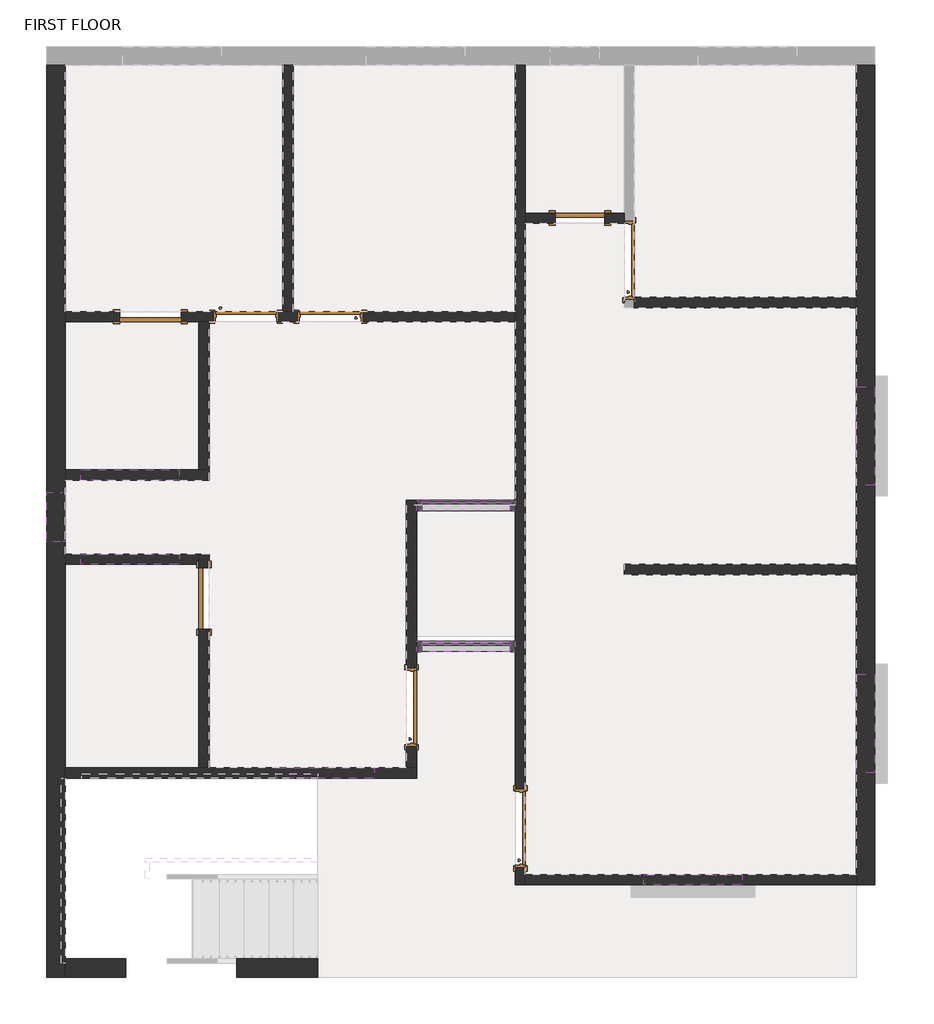
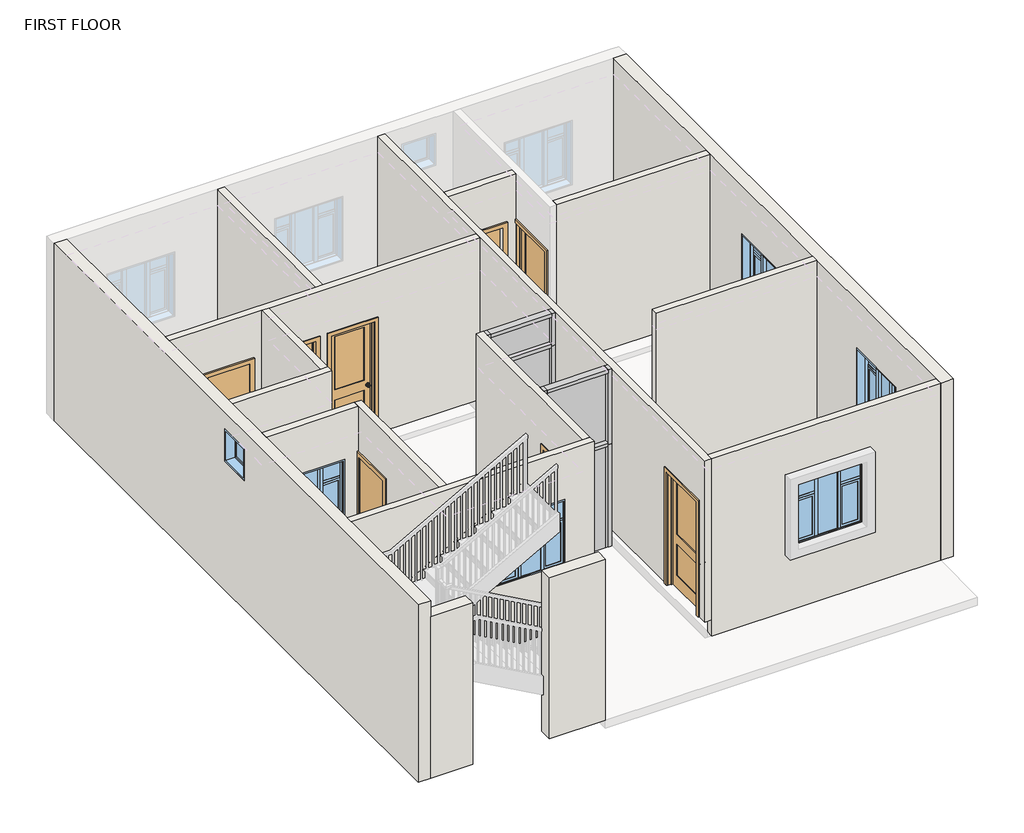
# One storey, part 1 of 3: 16 walls, 14 members, 8 doors, 7 windows, 4 plates.
"""IFC4 building model written with IfcOpenShell, lengths in millimetres."""

from ifc_helpers import new_model, si_unit, frame, origin, place, context, project, spatial, polyline, outline, extrude, faceted_brep, transform, mapped, element, save
from components import door_2e56f206, door_interior_single_2_panel_wood_main_doors_a5f98f63, door_interior_single_2_panel_wood_main_doors_4d656947, single_flush_bathroom_flush_door_4d6c7550, single_flush_bathroom_flush_door_2_931cabab, member_273a15f2, member_867fe1e1, member_ee409385, member_47bfaf8a, member_4b717c4e, system_panel_glazed_c5a9eb28, system_panel_glazed_3290db12, system_panel_glazed_e6353eef, fixed_opening_window_2_x_2_e119d648, window_casement_triple_side_transom_window_4_x_4_fd24aed3, window_casement_triple_side_transom_window_4_x_4_9406f89d

model = new_model("IFC4")

# Units and contexts
model_context = context("Model", 3, world=origin())
ifc_project = project(units=[si_unit("LENGTHUNIT", "METRE", prefix="MILLI")], contexts=[model_context])

# Site, building, storey
site = spatial("IfcSite", under=ifc_project)
building = spatial("IfcBuilding", under=site)
storey = spatial("IfcBuildingStorey", under=building, Name="FIRST FLOOR", Elevation=3352.8)

# Doors
placement = place(None, origin())
door_shape = door_2e56f206(model_context)
element("IfcDoor", 1, ObjectType="Door-Interior-Single-2_Panel-Wood : 36\" x 84\"", at=placement, inside=storey, context=model_context, shape_type="MappedRepresentation", body=[
    mapped(door_shape, transform((-9131.4273867, -1143.8499863, 3657.6), x_axis=(0.0, 1.0, 0.0), y_axis=(-1.0, 0.0, 0.0), z_axis=(0.0, 0.0, 1.0))),
])
element("IfcDoor", 2, ObjectType="Door-Interior-Single-2_Panel-Wood : 36\" x 84\"", at=placement, inside=storey, context=model_context, shape_type="MappedRepresentation", body=[
    mapped(door_shape, transform((-10477.6273867, 354.7500137, 3657.6), x_axis=(0.0, 1.0, 0.0), y_axis=(-1.0, 0.0, 0.0), z_axis=(0.0, 0.0, 1.0))),
])
element("IfcDoor", 3, ObjectType="Door-Interior-Single-2_Panel-Wood : 36\" x 84\"", at=placement, inside=storey, context=model_context, shape_type="MappedRepresentation", body=[
    mapped(door_shape, transform((-7785.2273867, 5879.2500137, 3657.6), x_axis=(0.0, 1.0, 0.0), y_axis=(-1.0, 0.0, 0.0), z_axis=(0.0, 0.0, 1.0))),
])
door_interior_single_2_panel_wood_main_doors_shape = door_interior_single_2_panel_wood_main_doors_a5f98f63(model_context)
element("IfcDoor", 4, ObjectType="Door-Interior-Single-2_Panel-Wood : MAIN DOORS", at=placement, inside=storey, context=model_context, shape_type="MappedRepresentation", body=[
    mapped(door_interior_single_2_panel_wood_main_doors_shape, transform((-12525.5023867, 5183.9250137, 3657.6), x_axis=(1.0, 0.0, 0.0), y_axis=(0.0, 1.0, 0.0), z_axis=(0.0, 0.0, 1.0))),
])
door_interior_single_2_panel_wood_main_doors_2_shape = door_interior_single_2_panel_wood_main_doors_4d656947(model_context)
element("IfcDoor", 5, ObjectType="Door-Interior-Single-2_Panel-Wood : MAIN DOORS", at=placement, inside=storey, context=model_context, shape_type="MappedRepresentation", body=[
    mapped(door_interior_single_2_panel_wood_main_doors_2_shape, transform((-11484.1023867, 5183.9250137, 3657.6), x_axis=(-1.0, 0.0, 0.0), y_axis=(0.0, -1.0, 0.0), z_axis=(0.0, 0.0, 1.0))),
])
single_flush_bathroom_flush_door_shape = single_flush_bathroom_flush_door_4d6c7550(model_context)
element("IfcDoor", 6, ObjectType="Single-Flush : BATHROOM FLUSH DOOR", at=placement, inside=storey, context=model_context, shape_type="MappedRepresentation", body=[
    mapped(single_flush_bathroom_flush_door_shape, transform((-13046.2023867, 1700.5265627, 3657.6), x_axis=(0.0, 1.0, 0.0), y_axis=(-1.0, 0.0, 0.0), z_axis=(0.0, 0.0, 1.0))),
])
element("IfcDoor", 7, ObjectType="Single-Flush : BATHROOM FLUSH DOOR", at=placement, inside=storey, context=model_context, shape_type="MappedRepresentation", body=[
    mapped(single_flush_bathroom_flush_door_shape, transform((-13706.6023867, 5180.7500137, 3657.6), x_axis=(-1.0, 0.0, 0.0), y_axis=(0.0, -1.0, 0.0), z_axis=(0.0, 0.0, 1.0))),
])
single_flush_bathroom_flush_door_2_shape = single_flush_bathroom_flush_door_2_931cabab(model_context)
element("IfcDoor", 8, ObjectType="Single-Flush : BATHROOM FLUSH DOOR 2", at=placement, inside=storey, context=model_context, shape_type="MappedRepresentation", body=[
    mapped(single_flush_bathroom_flush_door_2_shape, transform((-8398.0023867, 6399.9500137, 3657.6), x_axis=(-1.0, 0.0, 0.0), y_axis=(0.0, -1.0, 0.0), z_axis=(0.0, 0.0, 1.0))),
])

# Members
member_shape = member_273a15f2(model_context)
element("IfcMember", 9, ObjectType="Rectangular Mullion : 2.5\" x 5\" rectangular", at=placement, inside=storey, context=model_context, shape_type="MappedRepresentation", body=[
    mapped(member_shape, transform((-9261.6023867, 2848.1833471, 6705.6), x_axis=(0.0, 0.0, 1.0), y_axis=(0.0, -1.0, 0.0), z_axis=(1.0, 0.0, 0.0))),
])
element("IfcMember", 10, ObjectType="Rectangular Mullion : 2.5\" x 5\" rectangular", at=placement, inside=storey, context=model_context, shape_type="MappedRepresentation", body=[
    mapped(member_shape, transform((-9261.6023867, 1104.0500137, 6705.6), x_axis=(0.0, 0.0, 1.0), y_axis=(0.0, -1.0, 0.0), z_axis=(1.0, 0.0, 0.0))),
])
element("IfcMember", 11, ObjectType="Rectangular Mullion : 2.5\" x 5\" rectangular", at=placement, inside=storey, context=model_context, shape_type="MappedRepresentation", body=[
    mapped(member_shape, transform((-10353.8023867, 2848.1833471, 3657.6), x_axis=(0.0, 0.0, -1.0), y_axis=(0.0, -1.0, 0.0), z_axis=(-1.0, 0.0, 0.0))),
])
element("IfcMember", 12, ObjectType="Rectangular Mullion : 2.5\" x 5\" rectangular", at=placement, inside=storey, context=model_context, shape_type="MappedRepresentation", body=[
    mapped(member_shape, transform((-10353.8023867, 1104.0500137, 2851.15), x_axis=(0.0, 0.0, -1.0), y_axis=(0.0, -1.0, 0.0), z_axis=(-1.0, 0.0, 0.0))),
])
member_2_shape = member_867fe1e1(model_context)
element("IfcMember", 13, ObjectType="Rectangular Mullion : 2.5\" x 5\" rectangular", at=placement, inside=storey, context=model_context, shape_type="MappedRepresentation", body=[
    mapped(member_2_shape, transform((-9261.6023867, 2848.1833471, 6096.0), x_axis=(0.0, 0.0, 1.0), y_axis=(0.0, -1.0, 0.0), z_axis=(1.0, 0.0, 0.0))),
])
element("IfcMember", 14, ObjectType="Rectangular Mullion : 2.5\" x 5\" rectangular", at=placement, inside=storey, context=model_context, shape_type="MappedRepresentation", body=[
    mapped(member_2_shape, transform((-9261.6023867, 1104.0500137, 5289.55), x_axis=(0.0, 0.0, 1.0), y_axis=(0.0, -1.0, 0.0), z_axis=(1.0, 0.0, 0.0))),
])
member_3_shape = member_ee409385(model_context)
element("IfcMember", 15, ObjectType="Rectangular Mullion : 2.5\" x 5\" rectangular", at=placement, inside=storey, context=model_context, shape_type="MappedRepresentation", body=[
    mapped(member_3_shape, transform((-9198.1023867, 2848.1833471, 3657.6), x_axis=(1.0, 0.0, 0.0), y_axis=(0.0, -1.0, 0.0), z_axis=(0.0, 0.0, -1.0))),
])
element("IfcMember", 16, ObjectType="Rectangular Mullion : 2.5\" x 5\" rectangular", at=placement, inside=storey, context=model_context, shape_type="MappedRepresentation", body=[
    mapped(member_3_shape, transform((-9198.1023867, 1104.0500137, 2851.15), x_axis=(1.0, 0.0, 0.0), y_axis=(0.0, -1.0, 0.0), z_axis=(0.0, 0.0, -1.0))),
])
member_4_shape = member_47bfaf8a(model_context)
element("IfcMember", 17, ObjectType="Rectangular Mullion : 2.5\" x 5\" rectangular", at=placement, inside=storey, context=model_context, shape_type="MappedRepresentation", body=[
    mapped(member_4_shape, transform((-10417.3023867, 2848.1833471, 6705.6), x_axis=(-1.0, 0.0, 0.0), y_axis=(0.0, -1.0, 0.0), z_axis=(0.0, 0.0, 1.0))),
])
element("IfcMember", 18, ObjectType="Rectangular Mullion : 2.5\" x 5\" rectangular", at=placement, inside=storey, context=model_context, shape_type="MappedRepresentation", body=[
    mapped(member_4_shape, transform((-9198.1023867, 2848.1833471, 6096.0), x_axis=(1.0, 0.0, 0.0), y_axis=(0.0, -1.0, 0.0), z_axis=(0.0, 0.0, -1.0))),
])
element("IfcMember", 19, ObjectType="Rectangular Mullion : 2.5\" x 5\" rectangular", at=placement, inside=storey, context=model_context, shape_type="MappedRepresentation", body=[
    mapped(member_3_shape, transform((-10417.3023867, 2848.1833471, 6096.0), x_axis=(-1.0, 0.0, 0.0), y_axis=(0.0, -1.0, 0.0), z_axis=(0.0, 0.0, 1.0))),
])
element("IfcMember", 20, ObjectType="Rectangular Mullion : 2.5\" x 5\" rectangular", at=placement, inside=storey, context=model_context, shape_type="MappedRepresentation", body=[
    mapped(member_3_shape, transform((-10417.3023867, 1104.0500137, 5289.55), x_axis=(-1.0, 0.0, 0.0), y_axis=(0.0, -1.0, 0.0), z_axis=(0.0, 0.0, 1.0))),
])
member_5_shape = member_4b717c4e(model_context)
element("IfcMember", 21, ObjectType="Rectangular Mullion : 2.5\" x 5\" rectangular", at=placement, inside=storey, context=model_context, shape_type="MappedRepresentation", body=[
    mapped(member_5_shape, transform((-10417.3023867, 1104.0500137, 6705.6), x_axis=(-1.0, 0.0, 0.0), y_axis=(0.0, -1.0, 0.0), z_axis=(0.0, 0.0, 1.0))),
])
element("IfcMember", 22, ObjectType="Rectangular Mullion : 2.5\" x 5\" rectangular", at=placement, inside=storey, context=model_context, shape_type="MappedRepresentation", body=[
    mapped(member_5_shape, transform((-9198.1023867, 1104.0500137, 5289.55), x_axis=(1.0, 0.0, 0.0), y_axis=(0.0, -1.0, 0.0), z_axis=(0.0, 0.0, -1.0))),
])

# Plates
system_panel_glazed_shape = system_panel_glazed_c5a9eb28(model_context)
element("IfcPlate", 23, ObjectType="System Panel : Glazed", at=placement, inside=storey, context=model_context, shape_type="MappedRepresentation", body=[
    mapped(system_panel_glazed_shape, transform((-9807.7023867, 2848.1833471, 3721.1), x_axis=(1.0, 0.0, 0.0), y_axis=(0.0, 1.0, 0.0), z_axis=(0.0, 0.0, 1.0))),
])
element("IfcPlate", 24, ObjectType="System Panel : Glazed", at=placement, inside=storey, context=model_context, shape_type="MappedRepresentation", body=[
    mapped(system_panel_glazed_shape, transform((-9807.7023867, 1104.0500137, 2914.65), x_axis=(1.0, 0.0, 0.0), y_axis=(0.0, 1.0, 0.0), z_axis=(0.0, 0.0, 1.0))),
])
system_panel_glazed_2_shape = system_panel_glazed_3290db12(model_context)
element("IfcPlate", 25, ObjectType="System Panel : Glazed", at=placement, inside=storey, context=model_context, shape_type="MappedRepresentation", body=[
    mapped(system_panel_glazed_2_shape, transform((-9807.7023867, 2848.1833471, 6127.75), x_axis=(1.0, 0.0, 0.0), y_axis=(0.0, 1.0, 0.0), z_axis=(0.0, 0.0, 1.0))),
])
system_panel_glazed_3_shape = system_panel_glazed_e6353eef(model_context)
element("IfcPlate", 26, ObjectType="System Panel : Glazed", at=placement, inside=storey, context=model_context, shape_type="MappedRepresentation", body=[
    mapped(system_panel_glazed_3_shape, transform((-9807.7023867, 1104.0500137, 5321.3), x_axis=(1.0, 0.0, 0.0), y_axis=(0.0, 1.0, 0.0), z_axis=(0.0, 0.0, 1.0))),
])

# Walls
element("IfcWall", 27, at=placement, inside=storey, context=model_context, shape_type="Brep", body=[
    faceted_brep([(-4981.7023867, 8292.2500137, 3352.8), (-4981.7023867, -1715.3499863, 3352.8), (-4981.7023867, -1842.3499863, 3352.8), (-4981.7023867, -1842.3499863, 6705.6), (-4981.7023867, -1715.3499863, 6705.6), (-4981.7023867, 1993.0500137, 6705.6), (-4981.7023867, 2120.0500137, 6705.6), (-4981.7023867, 5295.0500137, 6705.6), (-4981.7023867, 5422.0500137, 6705.6), (-4981.7023867, 8292.2500137, 6705.6), (-4981.7023867, 3097.9500137, 5791.2), (-4981.7023867, 3097.9500137, 4572.0), (-4981.7023867, 4317.1500137, 4572.0), (-4981.7023867, 4317.1500137, 5791.2), (-4981.7023867, -458.0499863, 5791.2), (-4981.7023867, -458.0499863, 4572.0), (-4981.7023867, 761.1500137, 4572.0), (-4981.7023867, 761.1500137, 5791.2), (-4753.1023867, 8292.2500137, 3352.8), (-4753.1023867, 8292.2500137, 6705.6), (-4753.1023867, -1842.3499863, 6705.6), (-4753.1023867, -1842.3499863, 3352.8), (-4753.1023867, 3097.9500137, 5791.2), (-4753.1023867, 4317.1500137, 5791.2), (-4753.1023867, 4317.1500137, 4572.0), (-4753.1023867, 3097.9500137, 4572.0), (-4753.1023867, -458.0499863, 5791.2), (-4753.1023867, 761.1500137, 5791.2), (-4753.1023867, 761.1500137, 4572.0), (-4753.1023867, -458.0499863, 4572.0)], [[[0, 1, 2, 3, 4, 5, 6, 7, 8, 9], [10, 11, 12, 13], [14, 15, 16, 17]], [[18, 19, 20, 21], [22, 23, 24, 25], [26, 27, 28, 29]], [[2, 1, 0, 18, 21]], [[9, 8, 7, 6, 5, 4, 3, 20, 19]], [[0, 9, 19, 18]], [[3, 2, 21, 20]], [[11, 10, 22, 25]], [[12, 11, 25, 24]], [[13, 12, 24, 23]], [[10, 13, 23, 22]], [[15, 14, 26, 29]], [[16, 15, 29, 28]], [[17, 16, 28, 27]], [[14, 17, 27, 26]]]),
])
element("IfcWall", 28, at=placement, inside=storey, context=model_context, shape_type="Brep", body=[
    faceted_brep([(-14760.7023867, -2985.3499863, 3352.8), (-14760.7023867, -2756.7499863, 3352.8), (-14760.7023867, -521.5499863, 3352.8), (-14760.7023867, -394.5499863, 3352.8), (-14760.7023867, 8292.2500137, 3352.8), (-14760.7023867, 8292.2500137, 6705.6), (-14760.7023867, 5244.2500137, 6705.6), (-14760.7023867, 5117.2500137, 6705.6), (-14760.7023867, 3288.4500137, 6705.6), (-14760.7023867, 3161.4500137, 6705.6), (-14760.7023867, 2246.6265627, 6705.6), (-14760.7023867, 2119.6265627, 6705.6), (-14760.7023867, -394.5499863, 6705.6), (-14760.7023867, -521.5499863, 6705.6), (-14760.7023867, -2985.3499863, 6705.6), (-14760.7023867, -2985.3499863, 6400.8), (-14760.7023867, 2399.2382882, 5791.2), (-14760.7023867, 2399.2382882, 6400.8), (-14760.7023867, 3008.8382882, 6400.8), (-14760.7023867, 3008.8382882, 5791.2), (-14989.3023867, 8292.2500137, 3352.8), (-14989.3023867, -2985.3499863, 3352.8), (-14989.3023867, -2985.3499863, 6705.6), (-14989.3023867, 8292.2500137, 6705.6), (-14989.3023867, 2399.2382882, 6400.8), (-14989.3023867, 2399.2382882, 5791.2), (-14989.3023867, 3008.8382882, 5791.2), (-14989.3023867, 3008.8382882, 6400.8)], [[[0, 1, 2, 3, 4, 5, 6, 7, 8, 9, 10, 11, 12, 13, 14, 15], [16, 17, 18, 19]], [[20, 21, 22, 23], [24, 25, 26, 27]], [[4, 3, 2, 1, 0, 21, 20]], [[14, 13, 12, 11, 10, 9, 8, 7, 6, 5, 23, 22]], [[5, 4, 20, 23]], [[24, 17, 16, 25]], [[25, 16, 19, 26]], [[26, 19, 18, 27]], [[17, 24, 27, 18]], [[0, 15, 14, 22, 21]]]),
])
element("IfcWall", 29, at=placement, inside=storey, context=model_context, shape_type="SweptSolid", body=[
    extrude(outline(polyline([(-11636.5023867, -2756.7499863), (-11636.5023867, -2985.3499863), (-12639.8023867, -2985.3499863), (-12639.8023867, -2756.7499863), (-11636.5023867, -2756.7499863)])), frame((0.0, 0.0, 3352.8), z_axis=(0.0, 0.0, 1.0), x_axis=(1.0, 0.0, 0.0)), (0.0, 0.0, 1.0), 3048.0),
    extrude(outline(polyline([(-14760.7023867, -2985.3499863), (-14760.7023867, -2756.7499863), (-14011.4023867, -2756.7499863), (-14011.4023867, -2985.3499863), (-14760.7023867, -2985.3499863)])), frame((0.0, 0.0, 3352.8), z_axis=(0.0, 0.0, 1.0), x_axis=(1.0, 0.0, 0.0)), (0.0, 0.0, 1.0), 3048.0),
])
element("IfcWall", 30, ObjectType="INNER WALL 5\"", at=placement, inside=storey, context=model_context, shape_type="Brep", body=[
    faceted_brep([(-4981.7023867, 5422.0500137, 3657.6), (-7724.9023867, 5422.0500137, 3657.6), (-7724.9023867, 5422.0500137, 6705.6), (-4981.7023867, 5422.0500137, 6705.6), (-4981.7023867, 5295.0500137, 3657.6), (-4981.7023867, 5295.0500137, 6705.6), (-7724.9023867, 5295.0500137, 6705.6), (-7724.9023867, 5295.0500137, 3657.6), (-7724.9023867, 5396.6500137, 3657.6)], [[[0, 1, 2, 3]], [[4, 5, 6, 7]], [[1, 0, 4, 7, 8]], [[3, 2, 6, 5]], [[2, 1, 8, 7, 6]], [[0, 3, 5, 4]]]),
])
element("IfcWall", 31, ObjectType="INNER WALL 5\"", at=placement, inside=storey, context=model_context, shape_type="Brep", body=[
    faceted_brep([(-9198.1023867, -1842.3499863, 6705.6), (-9198.1023867, 5117.2500137, 6705.6), (-9198.1023867, 5244.2500137, 6705.6), (-9198.1023867, 8292.2500137, 6705.6), (-9198.1023867, 8292.2500137, 3657.6), (-9198.1023867, 5244.2500137, 3657.6), (-9198.1023867, 5117.2500137, 3657.6), (-9198.1023867, -661.2499863, 3657.6), (-9198.1023867, -661.2499863, 5816.6), (-9198.1023867, -1626.4499863, 5816.6), (-9198.1023867, -1626.4499863, 3657.6), (-9198.1023867, -1842.3499863, 3657.6), (-9071.1023867, 8292.2500137, 6705.6), (-9071.1023867, 6463.4500137, 6705.6), (-9071.1023867, 6336.4500137, 6705.6), (-9071.1023867, -1715.3499863, 6705.6), (-9071.1023867, -1842.3499863, 6705.6), (-9071.1023867, -1842.3499863, 3657.6), (-9071.1023867, -1626.4499863, 3657.6), (-9071.1023867, -1626.4499863, 5816.6), (-9071.1023867, -661.2499863, 5816.6), (-9071.1023867, -661.2499863, 3657.6), (-9071.1023867, 6336.4500137, 3657.6), (-9071.1023867, 6463.4500137, 3657.6), (-9071.1023867, 8292.2500137, 3657.6), (-9134.6023867, -1842.3499863, 6705.6)], [[[0, 1, 2, 3, 4, 5, 6, 7, 8, 9, 10, 11]], [[12, 13, 14, 15, 16, 17, 18, 19, 20, 21, 22, 23, 24]], [[4, 24, 23, 22, 21, 7, 6, 5]], [[17, 11, 10, 18]], [[3, 2, 1, 0, 25, 16, 15, 14, 13, 12]], [[4, 3, 12, 24]], [[0, 11, 17, 16, 25]], [[20, 8, 7, 21]], [[8, 20, 19, 9]], [[9, 19, 18, 10]]]),
])
element("IfcWall", 32, ObjectType="INNER WALL 5\"", at=placement, inside=storey, context=model_context, shape_type="Brep", body=[
    faceted_brep([(-9071.1023867, -1842.3499863, 3352.8), (-4981.7023867, -1842.3499863, 3352.8), (-4981.7023867, -1842.3499863, 6705.6), (-9071.1023867, -1842.3499863, 6705.6), (-9071.1023867, -1842.3499863, 3657.6), (-7610.6023867, -1842.3499863, 5791.2), (-6391.4023867, -1842.3499863, 5791.2), (-6391.4023867, -1842.3499863, 4572.0), (-7610.6023867, -1842.3499863, 4572.0), (-9071.1023867, -1715.3499863, 3352.8), (-9071.1023867, -1715.3499863, 6705.6), (-4981.7023867, -1715.3499863, 6705.6), (-4981.7023867, -1715.3499863, 3352.8), (-7610.6023867, -1715.3499863, 5791.2), (-7610.6023867, -1715.3499863, 4572.0), (-6391.4023867, -1715.3499863, 4572.0), (-6391.4023867, -1715.3499863, 5791.2)], [[[0, 1, 2, 3, 4], [5, 6, 7, 8]], [[9, 10, 11, 12], [13, 14, 15, 16]], [[1, 0, 9, 12]], [[3, 2, 11, 10]], [[0, 4, 3, 10, 9]], [[2, 1, 12, 11]], [[14, 13, 5, 8]], [[15, 14, 8, 7]], [[16, 15, 7, 6]], [[13, 16, 6, 5]]]),
])
element("IfcWall", 33, ObjectType="INNER WALL 5\"", at=placement, inside=storey, context=model_context, shape_type="SweptSolid", body=[
    extrude(outline(polyline([(-7851.9023867, 2120.0500137), (-4981.7023867, 2120.0500137), (-4981.7023867, 1993.0500137), (-7851.9023867, 1993.0500137), (-7851.9023867, 2120.0500137)])), frame((0.0, 0.0, 3657.6), z_axis=(0.0, 0.0, 1.0), x_axis=(1.0, 0.0, 0.0)), (0.0, 0.0, 1.0), 3048.0),
])
element("IfcWall", 34, ObjectType="INNER WALL 5\"", at=placement, inside=storey, context=model_context, shape_type="SweptSolid", body=[
    extrude(outline(polyline([(-12068.3023867, 5244.2500137), (-12068.3023867, 8292.2500137), (-11941.3023867, 8292.2500137), (-11941.3023867, 5244.2500137), (-12068.3023867, 5244.2500137)])), frame((0.0, 0.0, 3657.6), z_axis=(0.0, 0.0, 1.0), x_axis=(1.0, 0.0, 0.0)), (0.0, 0.0, 1.0), 3048.0),
])
element("IfcWall", 35, ObjectType="INNER WALL 5\"", at=placement, inside=storey, context=model_context, shape_type="Brep", body=[
    faceted_brep([(-14760.7023867, 5244.2500137, 6705.6), (-12068.3023867, 5244.2500137, 6705.6), (-11941.3023867, 5244.2500137, 6705.6), (-9198.1023867, 5244.2500137, 6705.6), (-9198.1023867, 5244.2500137, 3657.6), (-11077.7023867, 5244.2500137, 3657.6), (-11077.7023867, 5244.2500137, 5816.6), (-11890.5023867, 5244.2500137, 5816.6), (-11890.5023867, 5244.2500137, 3657.6), (-11941.3023867, 5244.2500137, 3657.6), (-12068.3023867, 5244.2500137, 3657.6), (-12119.1023867, 5244.2500137, 3657.6), (-12119.1023867, 5244.2500137, 5816.6), (-12931.9023867, 5244.2500137, 5816.6), (-12931.9023867, 5244.2500137, 3657.6), (-13325.6023867, 5244.2500137, 3657.6), (-13325.6023867, 5244.2500137, 5791.2), (-14087.6023867, 5244.2500137, 5791.2), (-14087.6023867, 5244.2500137, 3657.6), (-14760.7023867, 5244.2500137, 3657.6), (-9198.1023867, 5117.2500137, 6705.6), (-12982.7023867, 5117.2500137, 6705.6), (-13109.7023867, 5117.2500137, 6705.6), (-14760.7023867, 5117.2500137, 6705.6), (-14760.7023867, 5117.2500137, 3657.6), (-14087.6023867, 5117.2500137, 3657.6), (-14087.6023867, 5117.2500137, 5791.2), (-13325.6023867, 5117.2500137, 5791.2), (-13325.6023867, 5117.2500137, 3657.6), (-13109.7023867, 5117.2500137, 3657.6), (-12982.7023867, 5117.2500137, 3657.6), (-12931.9023867, 5117.2500137, 3657.6), (-12931.9023867, 5117.2500137, 5816.6), (-12119.1023867, 5117.2500137, 5816.6), (-12119.1023867, 5117.2500137, 3657.6), (-11890.5023867, 5117.2500137, 3657.6), (-11890.5023867, 5117.2500137, 5816.6), (-11077.7023867, 5117.2500137, 5816.6), (-11077.7023867, 5117.2500137, 3657.6), (-9198.1023867, 5117.2500137, 3657.6)], [[[0, 1, 2, 3, 4, 5, 6, 7, 8, 9, 10, 11, 12, 13, 14, 15, 16, 17, 18, 19]], [[20, 21, 22, 23, 24, 25, 26, 27, 28, 29, 30, 31, 32, 33, 34, 35, 36, 37, 38, 39]], [[24, 19, 18, 25]], [[4, 39, 38, 5]], [[28, 15, 14, 31, 30, 29]], [[34, 11, 10, 9, 8, 35]], [[3, 2, 1, 0, 23, 22, 21, 20]], [[0, 19, 24, 23]], [[4, 3, 20, 39]], [[26, 25, 18, 17]], [[27, 26, 17, 16]], [[28, 27, 16, 15]], [[33, 12, 11, 34]], [[12, 33, 32, 13]], [[13, 32, 31, 14]], [[7, 36, 35, 8]], [[36, 7, 6, 37]], [[37, 6, 5, 38]]]),
])
element("IfcWall", 36, ObjectType="INNER WALL 5\"", at=placement, inside=storey, context=model_context, shape_type="Brep", body=[
    faceted_brep([(-14760.7023867, 3161.4500137, 3657.6), (-12982.7023867, 3161.4500137, 3657.6), (-12982.7023867, 3161.4500137, 6705.6), (-14760.7023867, 3161.4500137, 6705.6), (-14570.2023867, 3161.4500137, 5791.2), (-13351.0023867, 3161.4500137, 5791.2), (-13351.0023867, 3161.4500137, 4572.0), (-14570.2023867, 3161.4500137, 4572.0), (-14760.7023867, 3288.4500137, 3657.6), (-14760.7023867, 3288.4500137, 6705.6), (-13109.7023867, 3288.4500137, 6705.6), (-12982.7023867, 3288.4500137, 6705.6), (-12982.7023867, 3288.4500137, 3657.6), (-13109.7023867, 3288.4500137, 3657.6), (-14570.2023867, 3288.4500137, 5791.2), (-14570.2023867, 3288.4500137, 4572.0), (-13351.0023867, 3288.4500137, 4572.0), (-13351.0023867, 3288.4500137, 5791.2)], [[[0, 1, 2, 3], [4, 5, 6, 7]], [[8, 9, 10, 11, 12, 13], [14, 15, 16, 17]], [[1, 0, 8, 13, 12]], [[3, 2, 11, 10, 9]], [[0, 3, 9, 8]], [[2, 1, 12, 11]], [[15, 14, 4, 7]], [[16, 15, 7, 6]], [[17, 16, 6, 5]], [[14, 17, 5, 4]]]),
])
element("IfcWall", 37, ObjectType="INNER WALL 5\"", at=placement, inside=storey, context=model_context, shape_type="SweptSolid", body=[
    extrude(outline(polyline([(-12982.7023867, 5117.2500137), (-12982.7023867, 3288.4500137), (-13109.7023867, 3288.4500137), (-13109.7023867, 5117.2500137), (-12982.7023867, 5117.2500137)])), frame((0.0, 0.0, 3657.6), z_axis=(0.0, 0.0, 1.0), x_axis=(1.0, 0.0, 0.0)), (0.0, 0.0, 1.0), 3048.0),
])
element("IfcWall", 38, ObjectType="INNER WALL 5\"", at=placement, inside=storey, context=model_context, shape_type="Brep", body=[
    faceted_brep([(-14760.7023867, -521.5499863, 3352.8), (-10417.3023867, -521.5499863, 3352.8), (-10417.3023867, -521.5499863, 6705.6), (-14760.7023867, -521.5499863, 6705.6), (-12157.2023867, -521.5499863, 5791.2), (-10938.0023867, -521.5499863, 5791.2), (-10938.0023867, -521.5499863, 4572.0), (-12157.2023867, -521.5499863, 4572.0), (-14760.7023867, -394.5499863, 3352.8), (-14760.7023867, -394.5499863, 6705.6), (-13109.7023867, -394.5499863, 6705.6), (-12982.7023867, -394.5499863, 6705.6), (-10544.3023867, -394.5499863, 6705.6), (-10417.3023867, -394.5499863, 6705.6), (-10417.3023867, -394.5499863, 3657.6), (-10417.3023867, -394.5499863, 3352.8), (-12157.2023867, -394.5499863, 5791.2), (-12157.2023867, -394.5499863, 4572.0), (-10938.0023867, -394.5499863, 4572.0), (-10938.0023867, -394.5499863, 5791.2)], [[[0, 1, 2, 3], [4, 5, 6, 7]], [[8, 9, 10, 11, 12, 13, 14, 15], [16, 17, 18, 19]], [[1, 0, 8, 15]], [[3, 2, 13, 12, 11, 10, 9]], [[0, 3, 9, 8]], [[2, 1, 15, 14, 13]], [[17, 16, 4, 7]], [[18, 17, 7, 6]], [[19, 18, 6, 5]], [[16, 19, 5, 4]]]),
])
element("IfcWall", 39, ObjectType="INNER WALL 5\"", at=placement, inside=storey, context=model_context, shape_type="SweptSolid", body=[
    extrude(outline(polyline([(2911.6833471, 6705.6), (2911.6833471, 3657.6), (837.3500137, 3657.6), (837.3500137, 5816.6), (-127.8499863, 5816.6), (-127.8499863, 3657.6), (-394.5499863, 3657.6), (-394.5499863, 6705.6), (2911.6833471, 6705.6)])), frame((-10544.3023867, 0.0, 0.0), z_axis=(1.0, 0.0, 0.0), x_axis=(0.0, 1.0, 0.0)), (0.0, 0.0, 1.0), 127.0),
])
element("IfcWall", 40, ObjectType="INNER WALL 5\"", at=placement, inside=storey, context=model_context, shape_type="Brep", body=[
    faceted_brep([(-12982.7023867, 2081.5265627, 5791.2), (-12982.7023867, 2081.5265627, 3657.6), (-12982.7023867, 2246.6265627, 3657.6), (-12982.7023867, 2246.6265627, 6705.6), (-12982.7023867, -394.5499863, 6705.6), (-12982.7023867, -394.5499863, 3657.6), (-12982.7023867, 1319.5265627, 3657.6), (-12982.7023867, 1319.5265627, 5791.2), (-13109.7023867, 2246.6265627, 3657.6), (-13109.7023867, 2119.6265627, 3657.6), (-13109.7023867, 2081.5265627, 3657.6), (-13109.7023867, 2081.5265627, 5791.2), (-13109.7023867, 1319.5265627, 5791.2), (-13109.7023867, 1319.5265627, 3657.6), (-13109.7023867, -394.5499863, 3657.6), (-13109.7023867, -394.5499863, 6705.6), (-13109.7023867, 2119.6265627, 6705.6), (-13109.7023867, 2246.6265627, 6705.6)], [[[0, 1, 2, 3, 4, 5, 6, 7]], [[8, 9, 10, 11, 12, 13, 14, 15, 16, 17]], [[6, 5, 14, 13]], [[2, 1, 10, 9, 8]], [[4, 3, 17, 16, 15]], [[5, 4, 15, 14]], [[3, 2, 8, 17]], [[11, 10, 1, 0]], [[12, 11, 0, 7]], [[13, 12, 7, 6]]]),
])
element("IfcWall", 41, ObjectType="INNER WALL 5\"", at=placement, inside=storey, context=model_context, shape_type="SweptSolid", body=[
    extrude(outline(polyline([(3657.6, -14760.7023867), (3657.6, -13109.7023867), (6705.6, -13109.7023867), (6705.6, -14760.7023867), (3657.6, -14760.7023867)]), holes=[polyline([(5791.2, -13351.0023867), (4572.0, -13351.0023867), (4572.0, -14570.2023867), (5791.2, -14570.2023867), (5791.2, -13351.0023867)])]), frame((0.0, 2119.6265627, 0.0), z_axis=(0.0, 1.0, 0.0), x_axis=(0.0, 0.0, 1.0)), (0.0, 0.0, 1.0), 127.0),
])
element("IfcWall", 42, ObjectType="INNER WALL 5\"", at=placement, inside=storey, context=model_context, shape_type="Brep", body=[
    faceted_brep([(-9071.1023867, 6336.4500137, 3657.6), (-8702.8023867, 6336.4500137, 3657.6), (-8702.8023867, 6336.4500137, 5791.2), (-8093.2023867, 6336.4500137, 5791.2), (-8093.2023867, 6336.4500137, 3657.6), (-7851.9023867, 6336.4500137, 3657.6), (-7851.9023867, 6336.4500137, 6705.6), (-9071.1023867, 6336.4500137, 6705.6), (-8702.8023867, 6463.4500137, 5791.2), (-8702.8023867, 6463.4500137, 3657.6), (-9071.1023867, 6463.4500137, 3657.6), (-9071.1023867, 6463.4500137, 6705.6), (-7851.9023867, 6463.4500137, 6705.6), (-7851.9023867, 6463.4500137, 3657.6), (-8093.2023867, 6463.4500137, 3657.6), (-8093.2023867, 6463.4500137, 5791.2), (-7851.9023867, 6361.8500137, 3657.6)], [[[0, 1, 2, 3, 4, 5, 6, 7]], [[8, 9, 10, 11, 12, 13, 14, 15]], [[14, 13, 16, 5, 4]], [[10, 9, 1, 0]], [[7, 6, 12, 11]], [[6, 5, 16, 13, 12]], [[0, 7, 11, 10]], [[2, 1, 9, 8]], [[3, 2, 8, 15]], [[4, 3, 15, 14]]]),
])

# Windows
fixed_opening_window_2_x_2_shape = fixed_opening_window_2_x_2_e119d648(model_context)
element("IfcWindow", 43, ObjectType="Fixed : opening window 2' x 2'", at=placement, inside=storey, context=model_context, shape_type="MappedRepresentation", body=[
    mapped(fixed_opening_window_2_x_2_shape, transform((-14875.0023867, 2665.9382882, 3657.6), x_axis=(0.0, -1.0, 0.0), y_axis=(1.0, 0.0, 0.0), z_axis=(0.0, 0.0, 1.0))),
])
window_casement_triple_side_transom_window_4_x_4_shape = window_casement_triple_side_transom_window_4_x_4_fd24aed3(model_context)
element("IfcWindow", 44, ObjectType="Window-Casement-Triple-Side-Transom : window 4' x 4'", at=placement, inside=storey, context=model_context, shape_type="MappedRepresentation", body=[
    mapped(window_casement_triple_side_transom_window_4_x_4_shape, transform((-4867.4023867, 3707.5500137, 3657.6), x_axis=(0.0, -1.0, 0.0), y_axis=(1.0, 0.0, 0.0), z_axis=(0.0, 0.0, 1.0))),
])
element("IfcWindow", 45, ObjectType="Window-Casement-Triple-Side-Transom : window 4' x 4'", at=placement, inside=storey, context=model_context, shape_type="MappedRepresentation", body=[
    mapped(window_casement_triple_side_transom_window_4_x_4_shape, transform((-4867.4023867, 151.5500137, 3657.6), x_axis=(0.0, -1.0, 0.0), y_axis=(1.0, 0.0, 0.0), z_axis=(0.0, 0.0, 1.0))),
])
window_casement_triple_side_transom_window_4_x_4_2_shape = window_casement_triple_side_transom_window_4_x_4_9406f89d(model_context)
element("IfcWindow", 46, ObjectType="Window-Casement-Triple-Side-Transom : window 4' x 4'", at=placement, inside=storey, context=model_context, shape_type="MappedRepresentation", body=[
    mapped(window_casement_triple_side_transom_window_4_x_4_2_shape, transform((-7001.0023867, -1778.8499863, 3657.6), x_axis=(-1.0, 0.0, 0.0), y_axis=(0.0, -1.0, 0.0), z_axis=(0.0, 0.0, 1.0))),
])
element("IfcWindow", 47, ObjectType="Window-Casement-Triple-Side-Transom : window 4' x 4'", at=placement, inside=storey, context=model_context, shape_type="MappedRepresentation", body=[
    mapped(window_casement_triple_side_transom_window_4_x_4_2_shape, transform((-11547.6023867, -458.0499863, 3657.6), x_axis=(-1.0, 0.0, 0.0), y_axis=(0.0, -1.0, 0.0), z_axis=(0.0, 0.0, 1.0))),
])
element("IfcWindow", 48, ObjectType="Window-Casement-Triple-Side-Transom : window 4' x 4'", at=placement, inside=storey, context=model_context, shape_type="MappedRepresentation", body=[
    mapped(window_casement_triple_side_transom_window_4_x_4_2_shape, transform((-13960.6023867, 3224.9500137, 3657.6), x_axis=(-1.0, 0.0, 0.0), y_axis=(0.0, -1.0, 0.0), z_axis=(0.0, 0.0, 1.0))),
])
element("IfcWindow", 49, ObjectType="Window-Casement-Triple-Side-Transom : window 4' x 4'", at=placement, inside=storey, context=model_context, shape_type="MappedRepresentation", body=[
    mapped(window_casement_triple_side_transom_window_4_x_4_2_shape, transform((-13960.6023867, 2183.1265627, 3657.6), x_axis=(1.0, 0.0, 0.0), y_axis=(0.0, 1.0, 0.0), z_axis=(0.0, 0.0, 1.0))),
])

save(model, "model.ifc")

# Revit data of these elements
# Type "Door-Interior-Single-2_Panel-Wood : 36\" x 84\""
#   Type Mark = "8"
#   Assembly Code = "C1020300"
#   Analytic Construction = "Wooden"
#   Top Rail = 0' - 4 11/16"
#   Thickness = 0' - 1 3/8"
#   Thermal Resistance (R) = 2.5876 (h·ft²·°F)/BTU
#   Swing Angle [instance default] = 90.00°
#   Stiles = 0' - 4 3/4"
#   Rough Width = 3' - 2"
#   Rough Height = 7' - 1"
#   Lock Rail = 0' - 7 1/2"
#   Height = 7' - 0"
#   Width = 3' - 0"
#   Heat Transfer Coefficient (U) = 0.3865 BTU/(h·ft²·°F)
#   Bottom Rail = 0' - 9 1/8"
#   Trim Material = Cherry
#   Panel Material = Cherry
#   Frame Material = Cherry
#   Door Handle Material = Aluminum
#   Visual Light Transmittance = 0
#   Solar Heat Gain Coefficient = 0
#   Wall Closure = (empty or 0)
#   Function = (empty or 0)
# Type "Door-Interior-Single-2_Panel-Wood : MAIN DOORS"
#   Type Mark = "10"
#   Assembly Code = "C1020300"
#   Analytic Construction = "Wooden"
#   Top Rail = 0' - 4 11/16"
#   Thickness = 0' - 1 3/8"
#   Thermal Resistance (R) = 2.5876 (h·ft²·°F)/BTU
#   Swing Angle [instance default] = 90.00°
#   Stiles = 0' - 4 3/4"
#   Rough Width = 2' - 8"
#   Rough Height = 7' - 1"
#   Lock Rail = 0' - 7 1/2"
#   Height = 7' - 0"
#   Width = 2' - 6"
#   Heat Transfer Coefficient (U) = 0.3865 BTU/(h·ft²·°F)
#   Bottom Rail = 0' - 9 1/8"
#   Trim Material = Cherry
#   Panel Material = Cherry
#   Frame Material = Cherry
#   Door Handle Material = Aluminum
#   Visual Light Transmittance = 0
#   Solar Heat Gain Coefficient = 0
#   Wall Closure = (empty or 0)
#   Function = (empty or 0)
# Type "Single-Flush : BATHROOM FLUSH DOOR"
#   Type Mark = "9"
#   Construction Type Id = "MDOOR"
#   Assembly Code = "C1020"
#   Analytic Construction = "Metal"
#   Thickness = 0' - 2"
#   Heat Transfer Coefficient (U) = 0.651978 BTU/(h·ft²·°F)
#   Height = 7' - 0"
#   Trim Projection Ext = 0' - 1"
#   Trim Projection Int = 0' - 1"
#   Trim Width = 0' - 3"
#   Width = 2' - 6"
#   Define Thermal Properties by = 1
#   Door Material = Door - Panel
#   Frame Material = Door - Frame
#   Visual Light Transmittance = 0
#   Solar Heat Gain Coefficient = 0
#   Function = (empty or 0)
#   Wall Closure = (empty or 0)
# Type "Single-Flush : BATHROOM FLUSH DOOR 2"
#   Type Mark = "11"
#   Construction Type Id = "MDOOR"
#   Assembly Code = "C1020"
#   Analytic Construction = "Metal"
#   Thickness = 0' - 2"
#   Heat Transfer Coefficient (U) = 0.651978 BTU/(h·ft²·°F)
#   Height = 7' - 0"
#   Trim Projection Ext = 0' - 1"
#   Trim Projection Int = 0' - 1"
#   Trim Width = 0' - 3"
#   Width = 2' - 0"
#   Define Thermal Properties by = 1
#   Door Material = Door - Panel
#   Frame Material = Door - Frame
#   Visual Light Transmittance = 0
#   Solar Heat Gain Coefficient = 0
#   Function = (empty or 0)
#   Wall Closure = (empty or 0)
# Type "Rectangular Mullion : 2.5\" x 5\" rectangular"
#   built-in parameter 1007304 = 0.416667 (stored number, unit not read)
#   built-in parameter 1007301 = 0.104167 (stored number, unit not read)
#   built-in parameter 1007300 = 0.104167 (stored number, unit not read)
# Type "System Panel : Glazed"
#   Construction Type Id = "GSP4R"
#   Analytic Construction = "1/8 in Pilkington single glazing"
#   Visual Light Transmittance = 0.9
#   Solar Heat Gain Coefficient = 0.86
#   Heat Transfer Coefficient (U) = 1.18115 BTU/(h·ft²·°F)
#   Define Thermal Properties by = 1
# Type
#   Assembly Code = "B2010"
#   Layers, outside or top first: 0' - 9" "OUTER WALL" (function 1)
# Type "INNER WALL 5\""
#   Assembly Code = "B2010"
#   Layers, outside or top first: 0' - 5" "OUTER WALL" (function 1)
# Type "Fixed : opening window 2' x 2'"
#   Type Mark = "18"
#   Construction Type Id = "GSP4R"
#   Assembly Code = "B2020100"
#   Analytic Construction = "1/8 in Pilkington single glazing"
#   Visual Light Transmittance = 0.9
#   Solar Heat Gain Coefficient = 0.78
#   Heat Transfer Coefficient (U) = 0.6496 BTU/(h·ft²·°F)
#   Height = 2' - 0"
#   Default Sill Height = 7' - 0"
#   Width = 2' - 0"
#   Window Inset = 0' - 0 3/4"
#   Define Thermal Properties by = 1
#   Glass Pane Material = Glass
#   Sash Material = Sash
#   Wall Closure = (empty or 0)
# Type "Window-Casement-Triple-Side-Transom : window 4' x 4'"
#   Type Mark = "22"
#   Fire Rating = "0.5h"
#   Assembly Code = "B2020100"
#   Analytic Construction = "Double glazing - domestic"
#   Window Width = 1' - 4"
#   Window Inset [instance default] = 0' - 0 5/8"
#   Wall Thickness [instance default] = 0' - 6"
#   Visual Light Transmittance = 0.81
#   Transom Height Ratio = 0.3
#   Thermal Resistance (R) = 1.8146 (h·ft²·°F)/BTU
#   Solar Heat Gain Coefficient = 0.76
#   Rough Width = 4' - 0 1/2"
#   Rough Height = 4' - 0 1/2"
#   Open Window Height = 2' - 9.6"
#   Heat Transfer Coefficient (U) = 0.5511 BTU/(h·ft²·°F)
#   Height = 4' - 0"
#   Transom Height = 1' - 2.4"
#   Frame Gap 3 [instance default] = 0' - 1 83/128"
#   Frame Gap 2 [instance default] = 0' - 0 5/8"
#   Frame Gap 1 = 0' - 1 51/128"
#   Default Sill Height = 3' - 0"
#   Width = 4' - 0"
#   Frame Material = Metal - Aluminum
#   Glass Panel Material = Glass
#   Wall Closure = (empty or 0)
# Elements 1, 2, 3 (IfcDoor, "Door-Interior-Single-2_Panel-Wood : 36\" x 84\"")
#   Swing Angle = 90.00°
#   Phase Created = New Construction
#   Materials on its faces: "Cherry", "Aluminum"
# Elements 4, 5 (IfcDoor, "Door-Interior-Single-2_Panel-Wood : MAIN DOORS")
#   Swing Angle = 90.00°
#   Phase Created = New Construction
#   Materials on its faces: "Cherry", "Aluminum"
# Elements 6, 7 (IfcDoor, "Single-Flush : BATHROOM FLUSH DOOR")
#   Phase Created = New Construction
#   Materials on its faces: "Door - Frame", "Door - Panel"
# Element 8 (IfcDoor, "Single-Flush : BATHROOM FLUSH DOOR 2")
#   Phase Created = New Construction
#   Materials on its faces: "Door - Frame", "Door - Panel"
# Elements 9, 10, 11, 12, 13, 14, 15, 16, 17, 18, 19, 20, 21, 22 (IfcMember, "Rectangular Mullion : 2.5\" x 5\" rectangular")
#   Phase Created = New Construction
#   Materials on its faces: "Aluminum"
# Elements 23, 24, 25, 26 (IfcPlate, "System Panel : Glazed")
#   Phase Created = New Construction
#   Materials on its faces: "Glass"
# Elements 27, 28 (IfcWall)
#   built-in parameter 1001111 = 0' - 0"
#   Top Offset = 1' - 0"
#   Base Offset = 0' - 0"
#   wall height = 11' - 0"
#   Phase Created = New Construction
#   Base Constraint = FIRST FLOOR
#   Top Constraint = Level 3
#   Materials on its faces: "OUTER WALL"
# Element 29 (IfcWall)
#   Top Offset = 0' - 0"
#   Base Offset = 0' - 0"
#   wall height = 10' - 0"
#   Phase Created = New Construction
#   Base Constraint = FIRST FLOOR
#   Top Constraint = Level 3
#   Materials on its faces: "OUTER WALL"
# Elements 30, 31, 33, 34, 35, 36, 37, 39, 40, 41, 42 (IfcWall, "INNER WALL 5\"")
#   built-in parameter 1001111 = 1' - 0"
#   Top Offset = 1' - 0"
#   Base Offset = 1' - 0"
#   wall height = 10' - 0"
#   Phase Created = New Construction
#   Base Constraint = FIRST FLOOR
#   Top Constraint = Level 3
#   Materials on its faces: "OUTER WALL"
# Elements 32, 38 (IfcWall, "INNER WALL 5\"")
#   built-in parameter 1001111 = 0' - 0"
#   Top Offset = 1' - 0"
#   Base Offset = 0' - 0"
#   wall height = 11' - 0"
#   Phase Created = New Construction
#   Base Constraint = FIRST FLOOR
#   Top Constraint = Level 3
#   Materials on its faces: "OUTER WALL"
# Element 43 (IfcWindow, "Fixed : opening window 2' x 2'")
#   Mark = "14"
#   Phase Created = New Construction
#   Materials on its faces: "Sash", "Glass"
# Element 44 (IfcWindow, "Window-Casement-Triple-Side-Transom : window 4' x 4'")
#   Mark = "21"
#   Window Inset = 0' - 0 5/8"
#   Frame Gap 3 = 0' - 1 83/128"
#   Frame Gap 2 = 0' - 0 5/8"
#   Phase Created = New Construction
#   Materials on its faces: "Metal - Aluminum", "Glass"
# Element 45 (IfcWindow, "Window-Casement-Triple-Side-Transom : window 4' x 4'")
#   Mark = "22"
#   Window Inset = 0' - 0 5/8"
#   Frame Gap 3 = 0' - 1 83/128"
#   Frame Gap 2 = 0' - 0 5/8"
#   Phase Created = New Construction
#   Materials on its faces: "Metal - Aluminum", "Glass"
# Element 46 (IfcWindow, "Window-Casement-Triple-Side-Transom : window 4' x 4'")
#   Mark = "19"
#   Window Inset = 0' - 0 5/8"
#   Frame Gap 3 = 0' - 1 83/128"
#   Frame Gap 2 = 0' - 0 5/8"
#   Phase Created = New Construction
#   Materials on its faces: "Metal - Aluminum", "Glass"
# Element 47 (IfcWindow, "Window-Casement-Triple-Side-Transom : window 4' x 4'")
#   Mark = "20"
#   Window Inset = 0' - 0 5/8"
#   Frame Gap 3 = 0' - 1 83/128"
#   Frame Gap 2 = 0' - 0 5/8"
#   Phase Created = New Construction
#   Materials on its faces: "Metal - Aluminum", "Glass"
# Element 48 (IfcWindow, "Window-Casement-Triple-Side-Transom : window 4' x 4'")
#   Mark = "23"
#   Window Inset = 0' - 0 5/8"
#   Frame Gap 3 = 0' - 1 83/128"
#   Frame Gap 2 = 0' - 0 5/8"
#   Phase Created = New Construction
#   Materials on its faces: "Metal - Aluminum", "Glass"
# Element 49 (IfcWindow, "Window-Casement-Triple-Side-Transom : window 4' x 4'")
#   Mark = "24"
#   Window Inset = 0' - 0 5/8"
#   Frame Gap 3 = 0' - 1 83/128"
#   Frame Gap 2 = 0' - 0 5/8"
#   Phase Created = New Construction
#   Materials on its faces: "Metal - Aluminum", "Glass"
# Materials
#   "Cherry": class "Wood", colour RGB 226 177 128, transparency 0, Description = "Prunus Serotina", Cost = 0
#   "Aluminum": class "Metal", colour RGB 247 247 247, transparency 0, Description = "Aluminum 6061", Cost = 0
#   "Door - Panel": class "Wood", colour RGB 210 159 95, transparency 0, Cost = 0
#   "Door - Frame": colour RGB 118 70 51, transparency 0, Cost = 0
#   "OUTER WALL": class "Generic", colour RGB 245 245 240, transparency 0, Cost = 0
#   "Glass": class "Glass", colour RGB 0 128 192, transparency 0.75, Description = "Soda Lime Glass", Cost = 0
#   "Sash": class "Wood", colour RGB 224 178 126, transparency 0, Cost = 0
#   "Metal - Aluminum": class "Metal", colour RGB 247 247 247, transparency 0
